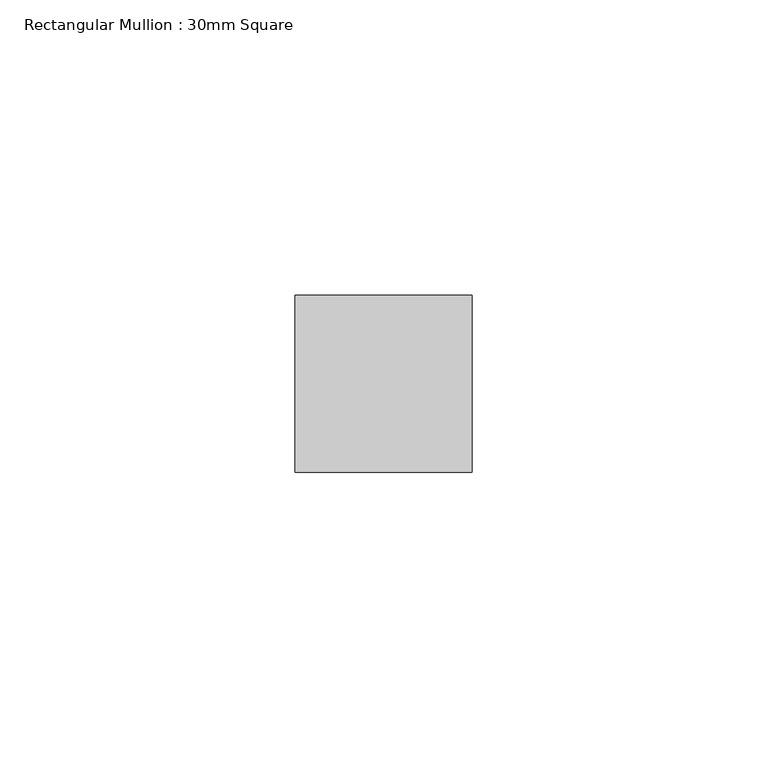
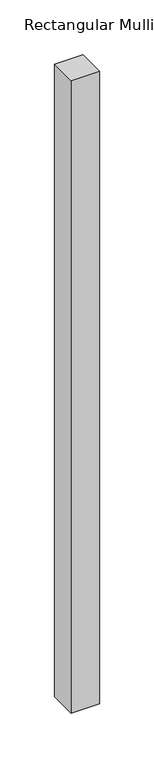
"""IFC4 building model written with IfcOpenShell, lengths in millimetres: member geometry, Rectangular Mullion : 30mm Square."""

from ifc_helpers import new_model, si_unit, frame, origin, place, context, project, spatial, polyline, outline, extrude, source, transform, mapped, element, save


def rectangular_mullion_30mm_square_a2edb205(model_context):
    return source(origin(), model_context, "Body", "SweptSolid", [
        extrude(outline(polyline([(0.0, 15.0), (0.0, -15.0), (-30.0, -15.0), (-30.0, 15.0), (0.0, 15.0)])), frame((0.0, 0.0, -705.0), z_axis=(0.0, 0.0, 1.0), x_axis=(1.0, 0.0, 0.0)), (0.0, 0.0, 1.0), 705.0),
    ])


if __name__ == "__main__":
    model = new_model("IFC4")
    model_context = context("Model", 3, world=origin())
    ifc_project = project(units=[si_unit("LENGTHUNIT", "METRE", prefix="MILLI")], contexts=[model_context])
    site = spatial("IfcSite", under=ifc_project)
    building = spatial("IfcBuilding", under=site)
    placement = place(None, origin())
    rectangular_mullion_30mm_square_shape = rectangular_mullion_30mm_square_a2edb205(model_context)
    element("IfcMember", 1, ObjectType="Rectangular Mullion : 30mm Square", at=placement, inside=building, context=model_context, shape_type="MappedRepresentation", body=[
        mapped(rectangular_mullion_30mm_square_shape, transform((0.0, 0.0, 0.0), x_axis=(1.0, 0.0, 0.0), y_axis=(0.0, 1.0, 0.0), z_axis=(0.0, 0.0, 1.0))),
    ])
    save(model, "model.ifc")

# Revit data of these elements
# Type "Rectangular Mullion : 30mm Square"
#   built-in parameter 1007304 = 0.0984252 (stored number, unit not read)
#   built-in parameter 1007301 = 0.0492126 (stored number, unit not read)
#   built-in parameter 1007300 = 0.0492126 (stored number, unit not read)
# Element 1 (IfcMember, "Rectangular Mullion : 30mm Square")
#   Materials on its faces: "Aluminum"
# Materials
#   "Aluminum": class "Metal", colour RGB 244 244 244, transparency 0, Description = "Aluminum 6061", Cost = 0
